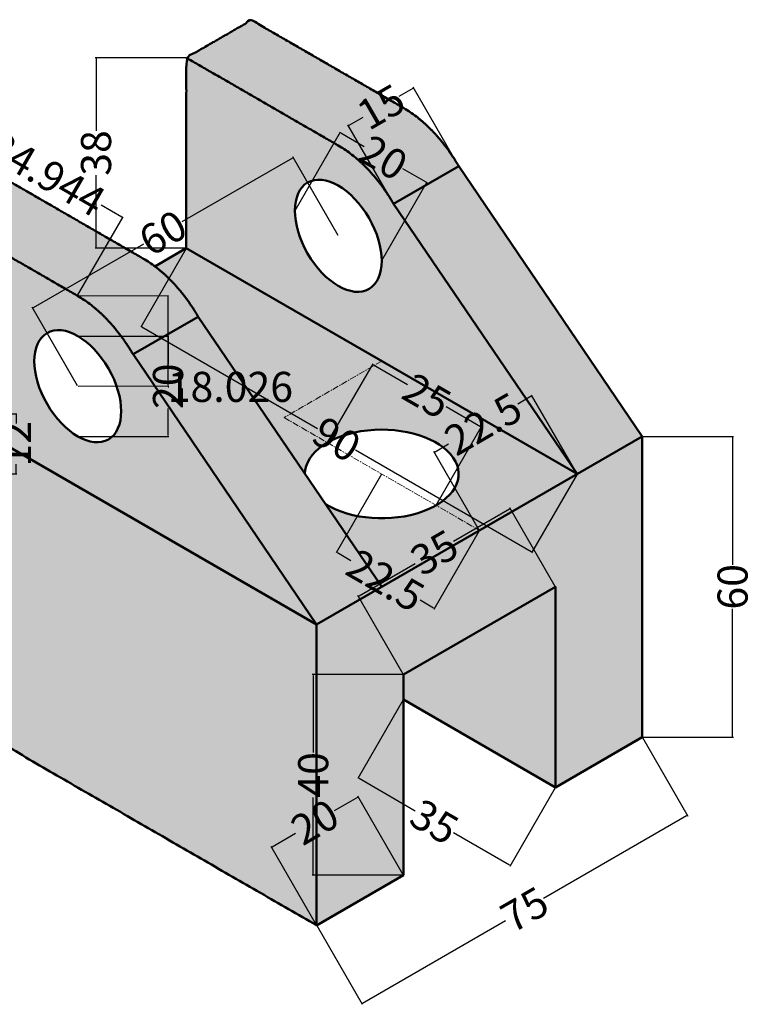
# Model space of a CAD drawing. Units: millimetres. Extents: x -57 to 165, y 2 to 198.
# Tile 1 of 1: x 18.8 to 164.9, y 1.8 to 198.1. Entities that reach past the tile are written whole.
import ezdxf

# ---------------------------------------------------------------- set-up
doc = ezdxf.new("R2010")
doc.units = ezdxf.units.MM
doc.header["$MEASUREMENT"] = 0
doc.linetypes.add('CENTER', pattern=[2, 1.25, -0.25, 0.25, -0.25])
for name, color, linetype, lineweight in [('M-CNTR', 7, 'CENTER', 18), ('M-DIMS', 2, 'Continuous', 18), ('M-HATC', 8, 'Continuous', 18), ('M-OUTL', 7, 'Continuous', 50)]:
    doc.layers.add(name, color=color, linetype=linetype, lineweight=lineweight)
doc.styles.get("Standard").update_dxf_attribs({"font": 'arial.ttf'})
doc.dimstyles.get("Standard").update_dxf_attribs({"dimtxt": 6, "dimasz": 0.18, "dimexe": 0.18, "dimexo": 0.0625, "dimgap": 0.09, "dimtad": 0, "dimtoh": 1, "dimdec": 0, "dimzin": 0, "dimdsep": 46, "dimtxsty": 'Standard', "dimcen": 0.09, "dimadec": 0, "dimazin": 0, "dimtfac": 1, "dimtdec": 0, "dimtofl": 0, "dimtmove": 0, "dimatfit": 3, "dimfxl": 1, "dimtolj": 1, "dimtzin": 0, "dimarcsym": 0})

# ---------------------------------------------------------------- blocks, each defined once
blk = doc.blocks.new('*D1')
at = {"layer": 'Defpoints', "color": 0, "transparency": 16777216}
for p in [(142.9404789999999, 54.99799699999999), (77.98857400000001, 17.497997), (86.98857372342155, 1.909540210928014)]:
    blk.add_point(p, dxfattribs=at)
at = {"layer": 'M-DIMS', "color": 0, "lineweight": -2, "transparency": 16777216}
for p, q in [((142.971729, 54.94387041226346), (152.0304787943798, 39.25365551534351)), ((151.7845942216985, 39.31954008802471), (123.2623607468992, 22.85222091346)), ((87.14445829610275, 1.999540210928017), (115.666691770902, 18.46685938549273)), ((78.01982400000001, 17.44387041226347), (87.07857372342156, 1.753655638246812))]:
    blk.add_line(p, q, dxfattribs=at)
at = {"layer": 'M-DIMS', "color": 0, "transparency": 16777216}
for points in [[(151.7695942216986, 39.34552085013825), (151.7995942216986, 39.29355932591118), (151.9404787943797, 39.40954008802471)], [(87.12945829610275, 2.025520973041551), (87.15945829610276, 1.973559448814484), (86.98857372342155, 1.909540210928014)]]:
    blk.add_solid(points, dxfattribs=at)
at = {"layer": 'M-DIMS', "color": 0, "transparency": 16777216, "insert": (119.4645262589006, 20.65954014947636), "char_height": 6, "attachment_point": 5, "rotation": 29.99999999999997}
blk.add_mtext('\\A1;75', dxfattribs=at)
blk = doc.blocks.new('*D2')
at = {"layer": 'Defpoints', "color": 0, "transparency": 16777216}
for p in [(52.007811, 152.497997), (43.00781132352439, 136.9095402922407), (129.9500979999999, 107.497997)]:
    blk.add_point(p, dxfattribs=at)
at = {"layer": 'M-DIMS', "color": 0, "lineweight": -2, "transparency": 16777216}
for p, q in [((51.976561, 152.4438704122635), (42.91781132352439, 136.7536557195595)), ((43.16369589620559, 136.8195402922407), (78.18820913771562, 116.5981281440193)), ((120.794213585993, 91.99954000671201), (85.76970034448304, 112.2209521549334)), ((129.9188479999999, 107.4438704122634), (120.8600981586743, 91.7536554340308))]:
    blk.add_line(p, q, dxfattribs=at)
at = {"layer": 'M-DIMS', "color": 0, "transparency": 16777216}
for points in [[(43.17869589620559, 136.8455210543543), (43.14869589620559, 136.7935595301272), (43.00781132352439, 136.9095402922407)], [(120.8092135859931, 92.02552076882554), (120.7792135859931, 91.97355924459848), (120.9500981586743, 91.909540006712)]]:
    blk.add_solid(points, dxfattribs=at)
at = {"layer": 'M-DIMS', "color": 0, "transparency": 16777216, "insert": (81.97895474109932, 114.4095401494764), "char_height": 6, "attachment_point": 5, "rotation": 330}
blk.add_mtext('\\A1;90', dxfattribs=at)
blk = doc.blocks.new('*D3')
at = {"layer": 'Defpoints', "color": 0, "transparency": 16777216}
for p in [(142.940479, 114.997997), (142.940479, 54.99799700000003), (160.9404790000001, 54.99799700000004)]:
    blk.add_point(p, dxfattribs=at)
at = {"layer": 'M-DIMS', "color": 0, "lineweight": -2, "transparency": 16777216}
for p, q in [((143.002979, 114.997997), (161.1204790000001, 114.997997)), ((160.9404790000001, 114.817997), (160.9404790000001, 89.39154406684862)), ((160.9404790000001, 55.17799700000003), (160.9404790000001, 80.60444993315147)), ((143.002979, 54.99799700000003), (161.1204790000001, 54.99799700000004))]:
    blk.add_line(p, q, dxfattribs=at)
at = {"layer": 'M-DIMS', "color": 0, "transparency": 16777216}
for points in [[(160.9104790000001, 114.817997), (160.9704790000001, 114.817997), (160.9404790000001, 114.997997)], [(160.9104790000001, 55.17799700000003), (160.9704790000001, 55.17799700000003), (160.9404790000001, 54.99799700000004)]]:
    blk.add_solid(points, dxfattribs=at)
at = {"layer": 'M-DIMS', "color": 0, "transparency": 16777216, "insert": (160.9404790000001, 84.99799699999996), "char_height": 6, "attachment_point": 5, "rotation": 90}
blk.add_mtext('\\A1;60', dxfattribs=at)
blk = doc.blocks.new('*D4')
at = {"layer": 'Defpoints', "color": 0, "transparency": 16777216}
for p in [(77.30908200000006, 67.49799700000003), (95.30908200000005, 67.49799700000003), (95.30908200000005, 27.49799700000002)]:
    blk.add_point(p, dxfattribs=at)
at = {"layer": 'M-DIMS', "color": 0, "lineweight": -2, "transparency": 16777216}
for p, q in [((95.24658200000002, 67.49799700000003), (77.12908200000007, 67.49799700000003)), ((77.30908200000006, 67.31799700000002), (77.30908200000006, 51.99590968758528)), ((77.30908200000007, 27.67799700000001), (77.30908200000006, 43.00008431241475)), ((95.24658200000002, 27.49799700000002), (77.12908200000008, 27.49799700000001))]:
    blk.add_line(p, q, dxfattribs=at)
at = {"layer": 'M-DIMS', "color": 0, "transparency": 16777216}
for points in [[(77.27908200000006, 67.31799700000002), (77.33908200000006, 67.31799700000002), (77.30908200000006, 67.49799700000003)], [(77.27908200000007, 27.67799700000001), (77.33908200000008, 27.67799700000001), (77.30908200000007, 27.49799700000001)]]:
    blk.add_solid(points, dxfattribs=at)
at = {"layer": 'M-DIMS', "color": 0, "transparency": 16777216, "insert": (77.30908200000006, 47.49799699999998), "char_height": 6, "attachment_point": 5, "rotation": 90}
blk.add_mtext('\\A1;40', dxfattribs=at)
blk = doc.blocks.new('*D5')
at = {"layer": 'Defpoints', "color": 0, "transparency": 16777216}
for p in [(116.6199710076562, 100.5864542548589), (125.619971, 84.99799699999998), (95.309082, 67.497997)]:
    blk.add_point(p, dxfattribs=at)
at = {"layer": 'M-DIMS', "color": 0, "lineweight": -2, "transparency": 16777216}
for p, q in [((116.464086434975, 100.4964542548589), (105.2818554117888, 94.04039016348177)), ((125.588721, 85.0521235877365), (116.5299710076562, 100.7423388275401)), ((86.4649665472236, 83.17645431221374), (97.6471975704098, 89.6325184035909)), ((95.277832, 67.5521235877365), (86.2190819745424, 83.24233888489493))]:
    blk.add_line(p, q, dxfattribs=at)
at = {"layer": 'M-DIMS', "color": 0, "transparency": 16777216}
for points in [[(116.449086434975, 100.5224350169724), (116.479086434975, 100.4704734927453), (116.6199710076562, 100.5864542548589)], [(86.4499665472236, 83.20243507432728), (86.4799665472236, 83.15047355010022), (86.3090819745424, 83.08645431221373)]]:
    blk.add_solid(points, dxfattribs=at)
at = {"layer": 'M-DIMS', "color": 0, "transparency": 16777216, "insert": (101.4645264910993, 91.83645428353631), "char_height": 6, "attachment_point": 5, "rotation": 30.000000000000025}
blk.add_mtext('\\A1;35', dxfattribs=at)
blk = doc.blocks.new('*D6')
at = {"layer": 'Defpoints', "color": 0, "transparency": 16777216}
for p in [(86.30908212556041, 43.08645405064289), (95.309082, 27.497997), (77.98857399999999, 17.497997)]:
    blk.add_point(p, dxfattribs=at)
at = {"layer": 'M-DIMS', "color": 0, "lineweight": -2, "transparency": 16777216}
for p, q in [((95.277832, 27.55212358773653), (86.2190821255604, 43.24233862332408)), ((86.1531975528792, 42.99645405064288), (81.483879248326, 40.30062187057703)), ((69.14445867931941, 33.17645408341707), (73.8137769838726, 35.87228626348291)), ((77.95732399999999, 17.55212358773652), (68.89857410663821, 33.24233865609827))]:
    blk.add_line(p, q, dxfattribs=at)
at = {"layer": 'M-DIMS', "color": 0, "transparency": 16777216}
for points in [[(86.1381975528792, 43.02243481275641), (86.1681975528792, 42.97047328852935), (86.30908212556041, 43.08645405064289)], [(69.12945867931943, 33.2024348455306), (69.15945867931941, 33.15047332130354), (68.98857410663821, 33.08645408341707)]]:
    blk.add_solid(points, dxfattribs=at)
at = {"layer": 'M-DIMS', "color": 0, "transparency": 16777216, "insert": (77.64882811609931, 38.08645406702998), "char_height": 6, "attachment_point": 5, "rotation": 30.000000000000025}
blk.add_mtext('\\A1;20', dxfattribs=at)
blk = doc.blocks.new('*D7')
at = {"layer": 'Defpoints', "color": 0, "transparency": 16777216}
for p in [(95.30908199999998, 62.497997), (86.30908197454241, 46.90953968778624), (125.619971, 44.99799699999999)]:
    blk.add_point(p, dxfattribs=at)
at = {"layer": 'M-DIMS', "color": 0, "lineweight": -2, "transparency": 16777216}
for p, q in [((95.277832, 62.44387041226346), (86.2190819745424, 46.75365511510503)), ((86.4649665472236, 46.81953968778624), (97.64719757040984, 40.3634755964091)), ((125.588721, 44.94387041226346), (116.5299710076562, 29.2536551724599)), ((116.464086434975, 29.49953974514112), (105.2818554117888, 35.95560383651826))]:
    blk.add_line(p, q, dxfattribs=at)
at = {"layer": 'M-DIMS', "color": 0, "transparency": 16777216}
for points in [[(86.4799665472236, 46.84552044989978), (86.4499665472236, 46.79355892567271), (86.30908197454241, 46.90953968778624)], [(116.479086434975, 29.52552050725465), (116.449086434975, 29.47355898302759), (116.6199710076562, 29.40953974514112)]]:
    blk.add_solid(points, dxfattribs=at)
at = {"layer": 'M-DIMS', "color": 0, "transparency": 16777216, "insert": (101.4645264910993, 38.15953971646368), "char_height": 6, "attachment_point": 5, "rotation": 330}
blk.add_mtext('\\A1;35', dxfattribs=at)
blk = doc.blocks.new('*D8')
at = {"layer": 'Defpoints', "color": 0, "transparency": 16777216}
for p in [(34.00781100000002, 190.497997), (52.00781100000003, 190.497997), (52.00781100000003, 152.497997)]:
    blk.add_point(p, dxfattribs=at)
at = {"layer": 'M-DIMS', "color": 0, "lineweight": -2, "transparency": 16777216}
for p, q in [((51.94531100000002, 190.497997), (33.82781100000002, 190.497997)), ((34.00781100000002, 190.317997), (34.00781100000003, 175.8894976821283)), ((34.00781100000003, 152.677997), (34.00781100000003, 167.1064963178718)), ((51.94531100000002, 152.497997), (33.82781100000002, 152.497997))]:
    blk.add_line(p, q, dxfattribs=at)
at = {"layer": 'M-DIMS', "color": 0, "transparency": 16777216}
for points in [[(33.97781100000002, 190.317997), (34.03781100000002, 190.317997), (34.00781100000002, 190.497997)], [(33.97781100000003, 152.677997), (34.03781100000003, 152.677997), (34.00781100000003, 152.497997)]]:
    blk.add_solid(points, dxfattribs=at)
at = {"layer": 'M-DIMS', "color": 0, "transparency": 16777216, "insert": (34.00781100000006, 171.497997), "char_height": 6, "attachment_point": 5, "rotation": 90}
blk.add_mtext('\\A1;38', dxfattribs=at)
blk = doc.blocks.new('*D9')
at = {"layer": 'Defpoints', "color": 0, "transparency": 16777216}
for p in [(97.33178524819515, 184.4504148382333), (106.331785, 168.861958), (93.341404, 161.3619579999999)]:
    blk.add_point(p, dxfattribs=at)
at = {"layer": 'M-DIMS', "color": 0, "lineweight": -2, "transparency": 16777216}
for p, q in [((106.300535, 168.9160845877365), (97.24178524819514, 184.6062994109145)), ((97.17590067551393, 184.3604148382333), (94.41112936372917, 182.7641733771266)), ((93.310154, 161.4160845877365), (84.25140423400347, 177.1062994354951)), ((84.49728880668468, 177.0404148628139), (87.2620601184694, 178.6366563239206))]:
    blk.add_line(p, q, dxfattribs=at)
at = {"layer": 'M-DIMS', "color": 0, "transparency": 16777216}
for points in [[(97.16090067551391, 184.3863956003468), (97.19090067551392, 184.3344340761197), (97.33178524819515, 184.4504148382333)], [(84.48228880668466, 177.0663956249274), (84.51228880668467, 177.0144341007004), (84.34140423400348, 176.9504148628139)]]:
    blk.add_solid(points, dxfattribs=at)
at = {"layer": 'M-DIMS', "color": 0, "transparency": 16777216, "insert": (90.8365947410993, 180.7004148505236), "char_height": 6, "attachment_point": 5, "rotation": 30.000000000000053}
blk.add_mtext('\\A1;15', dxfattribs=at)
blk = doc.blocks.new('*D10')
at = {"layer": 'Defpoints', "color": 0, "transparency": 16777216}
for p in [(73.31870089448267, 170.5864544508813), (82.318701, 154.997997), (30.35717600000001, 124.997997)]:
    blk.add_point(p, dxfattribs=at)
at = {"layer": 'M-DIMS', "color": 0, "lineweight": -2, "transparency": 16777216}
for p, q in [((73.16281632180147, 170.4964544508813), (51.14286186371283, 157.7832278169606)), ((82.28745099999999, 155.0521235877365), (73.22870089448267, 170.7423390235625)), ((21.51306066039725, 140.6764541161913), (43.53301511848588, 153.389680750112)), ((30.32592600000001, 125.0521235877365), (21.26717608771604, 140.7423386888725))]:
    blk.add_line(p, q, dxfattribs=at)
at = {"layer": 'M-DIMS', "color": 0, "transparency": 16777216}
for points in [[(73.14781632180149, 170.5224352129948), (73.17781632180149, 170.4704736887677), (73.31870089448267, 170.5864544508813)], [(21.49806066039725, 140.7024348783048), (21.52806066039725, 140.6504733540778), (21.35717608771605, 140.5864541161913)]]:
    blk.add_solid(points, dxfattribs=at)
at = {"layer": 'M-DIMS', "color": 0, "transparency": 16777216, "insert": (47.33793849109936, 155.5864542835363), "char_height": 6, "attachment_point": 5, "rotation": 29.999999999999883}
blk.add_mtext('\\A1;60', dxfattribs=at)
blk = doc.blocks.new('*D11')
at = {"layer": 'Defpoints', "color": 0, "transparency": 16777216}
for p in [(99.97895489336175, 165.586454083417), (73.658447, 159.997997), (90.97895499999998, 149.997997)]:
    blk.add_point(p, dxfattribs=at)
at = {"layer": 'M-DIMS', "color": 0, "lineweight": -2, "transparency": 16777216}
for p, q in [((73.689697, 160.0521235877365), (82.74844687443955, 175.742338623324)), ((82.81433144712074, 175.4964540506428), (87.48364975167397, 172.800621870577)), ((99.82307032068054, 165.676454083417), (95.15375201612736, 168.3722862634828)), ((91.01020499999998, 150.0521235877365), (100.0689548933617, 165.7423386560982))]:
    blk.add_line(p, q, dxfattribs=at)
at = {"layer": 'M-DIMS', "color": 0, "transparency": 16777216}
for points in [[(82.82933144712075, 175.5224348127563), (82.79933144712074, 175.4704732885293), (82.65844687443955, 175.5864540506428)], [(99.83807032068054, 165.7024348455306), (99.80807032068056, 165.6504733213035), (99.97895489336175, 165.586454083417)]]:
    blk.add_solid(points, dxfattribs=at)
at = {"layer": 'M-DIMS', "color": 0, "transparency": 16777216, "insert": (91.31870088390065, 170.5864540670299), "char_height": 6, "attachment_point": 5, "rotation": 330}
blk.add_mtext('\\A1;20', dxfattribs=at)
blk = doc.blocks.new('*D12')
at = {"layer": 'Defpoints', "color": 0, "transparency": 16777216}
for p in [(30.35717600000002, 134.997997), (30.35717600000002, 114.997997), (48.35717600000005, 114.997997)]:
    blk.add_point(p, dxfattribs=at)
at = {"layer": 'M-DIMS', "color": 0, "lineweight": -2, "transparency": 16777216}
for p, q in [((30.41967600000001, 134.997997), (48.53717600000006, 134.997997)), ((48.35717600000005, 134.817997), (48.35717600000005, 129.4263326070942)), ((48.35717600000005, 115.1779970000001), (48.35717600000005, 120.5696613929059)), ((30.41967600000001, 114.997997), (48.53717600000006, 114.997997))]:
    blk.add_line(p, q, dxfattribs=at)
at = {"layer": 'M-DIMS', "color": 0, "transparency": 16777216}
for points in [[(48.32717600000005, 134.817997), (48.38717600000006, 134.817997), (48.35717600000005, 134.997997)], [(48.32717600000005, 115.1779970000001), (48.38717600000006, 115.1779970000001), (48.35717600000005, 114.997997)]]:
    blk.add_solid(points, dxfattribs=at)
at = {"layer": 'M-DIMS', "color": 0, "transparency": 16777216, "insert": (48.35717600000008, 124.997997), "char_height": 6, "attachment_point": 5, "rotation": 90}
blk.add_mtext('\\A1;20', dxfattribs=at)
blk = doc.blocks.new('*D14')
at = {"layer": 'Defpoints', "color": 0, "transparency": 16777216}
for p in [(110.804272020727, 116.8364543040202), (80.15363699999999, 113.747997), (101.804272, 101.247997)]:
    blk.add_point(p, dxfattribs=at)
at = {"layer": 'M-DIMS', "color": 0, "lineweight": -2, "transparency": 16777216}
for p, q in [((80.184887, 113.8021235877365), (89.24363699707429, 129.4923388357336)), ((89.30952156975547, 129.2464542630524), (96.11554783821445, 125.316993164846)), ((110.6483874480458, 116.9264543040202), (103.8423611795868, 120.8559154022266)), ((101.835522, 101.3021235877365), (110.894272020727, 116.9923388767014))]:
    blk.add_line(p, q, dxfattribs=at)
at = {"layer": 'M-DIMS', "color": 0, "transparency": 16777216}
for points in [[(89.32452156975548, 129.272435025166), (89.29452156975547, 129.2204735009389), (89.15363699707429, 129.3364542630524)], [(110.6633874480458, 116.9524350661337), (110.6333874480458, 116.9004735419066), (110.804272020727, 116.8364543040202)]]:
    blk.add_solid(points, dxfattribs=at)
at = {"layer": 'M-DIMS', "color": 0, "transparency": 16777216, "insert": (99.97895450890066, 123.0864542835363), "char_height": 6, "attachment_point": 5, "rotation": 330}
blk.add_mtext('\\A1;25', dxfattribs=at)
blk = doc.blocks.new('*D15')
at = {"layer": 'Defpoints', "color": 0, "transparency": 16777216}
for p in [(90.97895499999998, 107.497997), (110.464526, 96.247997), (81.97895491795558, 91.909539589775)]:
    blk.add_point(p, dxfattribs=at)
at = {"layer": 'M-DIMS', "color": 0, "lineweight": -2, "transparency": 16777216}
for p, q in [((90.947705, 107.4438704122634), (81.88895491795557, 91.75365501709379)), ((110.433276, 96.19387041226346), (101.374526064243, 80.50365527047111)), ((82.13483949063676, 91.819539589775), (84.83138008985958, 90.26269114893294)), ((101.3086414915618, 80.74953984315232), (98.61210089233907, 82.30638828399435))]:
    blk.add_line(p, q, dxfattribs=at)
at = {"layer": 'M-DIMS', "color": 0, "transparency": 16777216}
for points in [[(82.14983949063677, 91.84552035188854), (82.11983949063676, 91.79355882766146), (81.97895491795558, 91.909539589775)], [(101.3236414915618, 80.77552060526585), (101.2936414915619, 80.72355908103879), (101.464526064243, 80.65953984315232)]]:
    blk.add_solid(points, dxfattribs=at)
at = {"layer": 'M-DIMS', "color": 0, "transparency": 16777216, "insert": (91.72174049109933, 86.28453971646366), "char_height": 6, "attachment_point": 5, "rotation": 330}
blk.add_mtext('\\A1;22.5', dxfattribs=at)
blk = doc.blocks.new('*D16')
at = {"layer": 'Defpoints', "color": 0, "transparency": 16777216}
for p in [(120.9500980642432, 123.0864541568477), (129.950098, 107.497997), (110.464526, 96.247997)]:
    blk.add_point(p, dxfattribs=at)
at = {"layer": 'M-DIMS', "color": 0, "lineweight": -2, "transparency": 16777216}
for p, q in [((120.794213491562, 122.9964541568477), (118.0976725173392, 121.4396054994993)), ((129.918848, 107.5521235877365), (120.8600980642432, 123.2423387295288)), ((110.433276, 96.30212358773655), (101.3745261679557, 111.9923385498936)), ((101.6204107406369, 111.9264539772125), (104.3169517148597, 113.4833026345608))]:
    blk.add_line(p, q, dxfattribs=at)
at = {"layer": 'M-DIMS', "color": 0, "transparency": 16777216}
for points in [[(120.779213491562, 123.0224349189612), (120.809213491562, 122.9704733947341), (120.9500980642432, 123.0864541568477)], [(101.6054107406369, 111.952434739326), (101.6354107406369, 111.9004732150989), (101.4645261679557, 111.8364539772124)]]:
    blk.add_solid(points, dxfattribs=at)
at = {"layer": 'M-DIMS', "color": 0, "transparency": 16777216, "insert": (111.2073121160994, 117.4614540670301), "char_height": 6, "attachment_point": 5, "rotation": 29.999999999999538}
blk.add_mtext('\\A1;22.5', dxfattribs=at)
blk = doc.blocks.new('*D17')
at = {"layer": 'Defpoints', "color": 0, "transparency": 16777216}
for p in [(0.0462869999999924, 160.497997), (39.30844832468702, 158.6118924312673), (30.307407, 143.024036)]:
    blk.add_point(p, dxfattribs=at)
at = {"layer": 'M-DIMS', "color": 0, "lineweight": -2, "transparency": 16777216}
for p, q in [((0.0775406150812756, 160.5521215004074), (9.137338633268897, 176.2417318143229)), ((9.203206783008142, 175.9958428417155), (13.32703206028853, 173.6145839495605)), ((39.1525697635137, 158.7019028427014), (35.0287444862333, 161.0831617348563)), ((30.33866061508128, 143.0781605004074), (39.39845873612112, 158.7677709924407))]:
    blk.add_line(p, q, dxfattribs=at)
at = {"layer": 'M-DIMS', "color": 0, "transparency": 16777216}
for points in [[(9.218208518247167, 176.021822601911), (9.18820504776913, 175.9698630815199), (9.047328221834803, 176.0858532531495)], [(39.16757149875272, 158.727882602897), (39.13756802827469, 158.6759230825059), (39.30844832468702, 158.6118924312673)]]:
    blk.add_solid(points, dxfattribs=at)
at = {"layer": 'M-DIMS', "color": 0, "transparency": 16777216, "insert": (24.17788827326091, 167.3488728422084), "char_height": 6, "attachment_point": 5, "rotation": 329.9961731765761}
blk.add_mtext('\\A1;34.944', dxfattribs=at)
blk = doc.blocks.new('*D18')
at = {"layer": 'Defpoints', "color": 0, "transparency": 16777216}
for p in [(30.307407, 143.024036), (30.357176, 124.997997), (48.35710765869329, 125.0476942343873)]:
    blk.add_point(p, dxfattribs=at)
at = {"layer": 'M-DIMS', "color": 0, "lineweight": -2, "transparency": 16777216}
for p, q in [((30.36990676178436, 143.0242085598391), (48.48733765671476, 143.0742302058516)), ((48.30783531511237, 142.8937339195761), (48.35661068635673, 125.2276935483263)), ((30.41967576178436, 124.998169559839), (48.53710697263225, 125.0481912067239)), ((48.35710765869329, 125.0476942343873), (48.35760463102985, 124.8676949204483)), ((48.35760463102985, 124.8676949204483), (48.53760463102986, 124.8676949204483))]:
    blk.add_line(p, q, dxfattribs=at)
at = {"layer": 'M-DIMS', "color": 0, "transparency": 16777216}
for points in [[(48.33783520076885, 142.8938167482989), (48.27783542945587, 142.8936510908533), (48.3073383427758, 143.073733233515)], [(48.38661057201322, 125.227776377049), (48.32661080070024, 125.2276107196035), (48.35710765869329, 125.0476942343873)]]:
    blk.add_solid(points, dxfattribs=at)
at = {"layer": 'M-DIMS', "color": 0, "transparency": 16777216, "insert": (60.79745456281703, 124.8676949204483), "char_height": 6, "attachment_point": 5}
blk.add_mtext('\\A1;18.026', dxfattribs=at)
blk = doc.blocks.new('*D19')
at = {"layer": 'Defpoints', "color": 0, "transparency": 16777216}
for p in [(0.046287, 119.497997), (0.046287, 107.497997), (18.04628700000001, 107.497997)]:
    blk.add_point(p, dxfattribs=at)
at = {"layer": 'M-DIMS', "color": 0, "lineweight": -2, "transparency": 16777216}
for p, q in [((0.108787, 119.497997), (18.22628700000001, 119.497997)), ((18.04628700000001, 119.317997), (18.04628700000001, 117.5723080504775)), ((18.04628700000001, 107.677997), (18.04628700000001, 109.4236859495225)), ((0.108787, 107.497997), (18.22628700000001, 107.497997))]:
    blk.add_line(p, q, dxfattribs=at)
at = {"layer": 'M-DIMS', "color": 0, "transparency": 16777216}
for points in [[(18.01628700000001, 119.317997), (18.07628700000001, 119.317997), (18.04628700000001, 119.497997)], [(18.01628700000001, 107.677997), (18.07628700000001, 107.677997), (18.04628700000001, 107.497997)]]:
    blk.add_solid(points, dxfattribs=at)
at = {"layer": 'M-DIMS', "color": 0, "transparency": 16777216, "insert": (18.04628700000004, 113.497997), "char_height": 6, "attachment_point": 5, "rotation": 90}
blk.add_mtext('\\A1;12', dxfattribs=at)

msp = doc.modelspace()

# ---------------------------------------------------------------- hatches: boundary and pattern name
at = {"layer": 'M-HATC'}
h = msp.add_hatch(color=256, dxfattribs=at)
h.set_gradient(color1=(16, 86, 137), color2=(147, 149, 152), tint=1)
h.paths.add_polyline_path([(95.30908161067455, 67.49799706451296), (125.6199707431299, 84.99799706451296), (125.6199707431299, 44.99799706451294), (142.9404788188187, 54.99799706451296), (142.9404788188187, 114.9979970645127), (77.98857353498579, 77.49799706451294), (77.98857353498579, 17.49799706451294), (95.30908161067455, 27.49799706451294)])
edge = h.paths.add_edge_path()
edge.add_spline(control_points=[(41.37988016936596, 131.3619580951918), (36.81412674377037, 139.2700750031551), (30.35717632684165, 142.9979970645129)], knot_values=[0, 0, 0, 0.7853981633974488, 0.7853981633974488, 0.7853981633974488], weights=[1, 0.9238795325112866, 1], degree=2, periodic=0)
edge.add_spline(control_points=[(30.35717632684165, 142.9979970645129), (15.20173176061398, 151.7479970645129), (0.0462871943863021, 160.4979970645129)], knot_values=[0.7853981633974488, 0.7853981633974488, 0.7853981633974488, 1.785398163397448, 1.785398163397448, 1.785398163397448], weights=[1, 1, 1], degree=2, periodic=0)
edge.add_spline(control_points=[(0.046287194386295, 160.4979970645129), (0.046287194386295, 147.4979970645129), (0.046287194386295, 134.4979970645129)], knot_values=[2.785398163397448, 2.785398163397448, 2.785398163397448, 3.419544504860864, 3.419544504860864, 3.419544504860864], weights=[1, 1, 1], degree=2, periodic=0)
edge.add_spline(control_points=[(0.046287194386295, 134.4979970645129), (0.046287194386295, 126.9979970645129), (0.046287194386295, 119.4979970645129)], knot_values=[3.419544504860864, 3.419544504860864, 3.419544504860864, 3.785398163397448, 3.785398163397448, 3.785398163397448], weights=[1, 1, 1], degree=2, periodic=0)
edge.add_spline(control_points=[(0.046287194386295, 119.4979970645129), (6.541477722769585, 123.2479970645129), (13.03666825115288, 126.9979970645129)], knot_values=[3, 3, 3, 4, 4, 4], weights=[1, 1, 1], degree=2, periodic=0)
edge.add_spline(control_points=[(13.03666825115288, 126.9979970645129), (13.03666825115288, 90.99799706451292), (13.03666825115288, 54.99799706451296)], knot_values=[2, 2, 2, 3, 3, 3], weights=[1, 1, 1], degree=2, periodic=0)
edge.add_line((13.03666825115287, 114.9979970645129), (77.98857353498579, 77.49799706451294))
edge.add_line((77.98857353498579, 77.49799706451294), (41.37988016936608, 131.3619580951916))
edge = h.paths.add_edge_path(flags=16)
edge.add_ellipse((30.35717632684166, 124.9979970645129), major_axis=(6.123724356957944, -10.60660171779821), ratio=0.577350269189626, start_angle=0, end_angle=360)
h.paths.add_polyline_path([(54.37026122613253, 138.8619580951918), (41.37988016936596, 131.3619580951918), (77.98857353498579, 77.49799706451294), (90.97895459175238, 84.99799706451292)])
edge = h.paths.add_edge_path()
edge.add_spline(control_points=[(45.75812342050349, 148.8897380148136), (44.56013330857391, 149.7979160278211), (43.34755738360823, 150.4979970645129)], knot_values=[0.6281854185381637, 0.6281854185381637, 0.6281854185381637, 0.7853981633974488, 0.7853981633974488, 0.7853981633974488], weights=[0.975625973363323, 0.9847630053244513, 1], degree=2, periodic=0)
edge.add_spline(control_points=[(43.34755738360823, 150.4979970645129), (28.19211281738056, 159.2479970645129), (13.03666825115287, 167.9979970645129)], knot_values=[0.7853981633974488, 0.7853981633974488, 0.7853981633974488, 1.785398163397448, 1.785398163397448, 1.785398163397448], weights=[1, 1, 1], degree=2, periodic=0)
edge.add_spline(control_points=[(13.03666825115287, 167.9979970645129), (6.541477722769585, 164.2479970645129), (0.046287194386295, 160.4979970645129)], knot_values=[1.785398163397448, 1.785398163397448, 1.785398163397448, 2.785398163397448, 2.785398163397448, 2.785398163397448], weights=[1, 1, 1], degree=2, periodic=0)
edge.add_spline(control_points=[(0.0462871943863021, 160.4979970645129), (15.20173176061398, 151.7479970645129), (30.35717632684165, 142.9979970645129)], knot_values=[0.7853981633974488, 0.7853981633974488, 0.7853981633974488, 1.785398163397448, 1.785398163397448, 1.785398163397448], weights=[1, 1, 1], degree=2, periodic=0)
edge.add_spline(control_points=[(30.35717632684165, 142.9979970645129), (36.81412674377037, 139.2700750031551), (41.37988016936596, 131.3619580951918)], knot_values=[0, 0, 0, 0.7853981633974488, 0.7853981633974488, 0.7853981633974488], weights=[1, 0.9238795325112866, 1], degree=2, periodic=0)
edge.add_line((41.37988016936598, 131.3619580951918), (54.37026122613254, 138.8619580951918))
edge.add_spline(control_points=[(54.37026122613254, 138.8619580951918), (50.7776825657607, 145.0844868651436), (45.75812342050349, 148.8897380148136)], knot_values=[0, 0, 0, 0.6281854185381637, 0.6281854185381637, 0.6281854185381637], weights=[1, 0.9391165271868352, 0.975625973363323], degree=2, periodic=0)
edge = h.paths.add_edge_path()
edge.add_spline(control_points=[(95.30908161067462, 180.4979970645128), (80.15363704444697, 189.2479970645128), (64.9981924782193, 197.9979970645128)], knot_values=[0.7853981633974488, 0.7853981633974488, 0.7853981633974488, 1.785398163397448, 1.785398163397448, 1.785398163397448], weights=[1, 1, 1], degree=2, periodic=0)
edge.add_spline(control_points=[(64.9981924782193, 197.9979970645128), (58.503001949836, 194.2479970645128), (52.0078114214527, 190.4979970645127)], knot_values=[1.785398163397448, 1.785398163397448, 1.785398163397448, 2.785398163397447, 2.785398163397448, 2.785398163397448], weights=[1, 1, 1], degree=2, periodic=0)
edge.add_spline(control_points=[(52.00781142145273, 190.4979970645127), (67.1632559876804, 181.7479970645128), (82.31870055390804, 172.9979970645128)], knot_values=[0.7853981633974488, 0.7853981633974488, 0.7853981633974488, 1.785398163397448, 1.785398163397448, 1.785398163397448], weights=[1, 1, 1], degree=2, periodic=0)
edge.add_spline(control_points=[(82.31870055390804, 172.9979970645128), (88.77565097083676, 169.2700750031549), (93.34140439643235, 161.3619580951917)], knot_values=[0, 0, 0, 0.7853981633974488, 0.7853981633974488, 0.7853981633974488], weights=[1, 0.9238795325112866, 1], degree=2, periodic=0)
edge.add_line((93.34140439643235, 161.3619580951917), (106.3317854531989, 168.8619580951917))
edge.add_spline(control_points=[(106.3317854531989, 168.8619580951917), (101.7660320276033, 176.7700750031549), (95.30908161067462, 180.4979970645128)], knot_values=[0, 0, 0, 0.7853981633974488, 0.7853981633974488, 0.7853981633974488], weights=[1, 0.9238795325112866, 1], degree=2, periodic=0)
h.paths.add_polyline_path([(106.3317854531989, 168.8619580951917), (93.34140439643235, 161.3619580951917), (129.9500977620521, 107.4979970645128), (142.9404788188187, 114.9979970645128)])
edge = h.paths.add_edge_path()
edge.add_spline(control_points=[(93.34140439643235, 161.3619580951917), (88.77565097083676, 169.2700750031549), (82.31870055390804, 172.9979970645128)], knot_values=[0, 0, 0, 0.7853981633974488, 0.7853981633974488, 0.7853981633974488], weights=[1, 0.9238795325112866, 1], degree=2, periodic=0)
edge.add_spline(control_points=[(82.31870055390804, 172.9979970645128), (67.1632559876804, 181.7479970645128), (52.00781142145273, 190.4979970645127)], knot_values=[0.7853981633974488, 0.7853981633974488, 0.7853981633974488, 1.785398163397448, 1.785398163397448, 1.785398163397448], weights=[1, 1, 1], degree=2, periodic=0)
edge.add_spline(control_points=[(52.0078114214527, 190.4979970645127), (52.0078114214527, 171.4979970645128), (52.0078114214527, 152.4979970645128)], knot_values=[2.785398163397447, 2.785398163397448, 2.785398163397448, 3.785398163397448, 3.785398163397448, 3.785398163397448], weights=[1, 1, 1], degree=2, periodic=0)
edge.add_line((52.0078114214527, 152.4979970645128), (129.9500977620521, 107.4979970645128))
edge.add_line((129.9500977620521, 107.4979970645128), (93.34140439643232, 161.3619580951917))
edge = h.paths.add_edge_path(flags=16)
edge.add_ellipse((82.31870055390804, 154.9979970645128), major_axis=(6.123724356957944, -10.60660171779821), ratio=0.577350269189626, start_angle=0, end_angle=360)
edge = h.paths.add_edge_path()
edge.add_line((52.0078114214527, 152.4979970645128), (45.7581234205035, 148.8897380148136))
edge.add_spline(control_points=[(45.75812342050349, 148.8897380148136), (50.7776825657607, 145.0844868651436), (54.37026122613254, 138.8619580951918)], knot_values=[0, 0, 0, 0.6281854185381637, 0.6281854185381637, 0.6281854185381637], weights=[0.975625973363323, 0.9391165271868352, 1], degree=2, periodic=0)
edge.add_line((54.37026122613257, 138.8619580951917), (75.66970573764932, 107.5231600210469))
edge.add_ellipse((90.97895459175238, 107.4979970645129), major_axis=(-15.30931089239486, 0), ratio=0.577350269189626, start_angle=330, end_angle=359.90582621493047, ccw=False)
edge.add_line((80.1536370444469, 113.7479970645129), (71.49338300660253, 118.7479970645128))
edge.add_line((71.49338300660253, 118.7479970645128), (90.97895459175236, 129.9979970645128))
edge.add_line((90.97895459175236, 129.9979970645128), (52.0078114214527, 152.4979970645128))
edge = h.paths.add_edge_path()
edge.add_line((90.97895459175236, 129.9979970645128), (71.49338300660254, 118.7479970645128))
edge.add_line((71.49338300660254, 118.7479970645128), (80.15363704444688, 113.7479970645129))
edge.add_ellipse((90.97895459175238, 107.4979970645129), major_axis=(-15.30931089239486, 0), ratio=0.577350269189626, start_angle=150.0000000000001, end_angle=330, ccw=False)
edge.add_line((101.8042721390579, 101.2479970645129), (110.4645261769023, 96.24799706451292))
edge.add_line((110.4645261769023, 96.24799706451292), (129.9500977620521, 107.4979970645128))
edge.add_line((129.9500977620521, 107.4979970645128), (90.97895459175236, 129.9979970645128))
edge = h.paths.add_edge_path(flags=17)
edge.add_line((110.4645261769023, 96.24799706451292), (101.8042721390579, 101.2479970645129))
edge.add_ellipse((90.97895459175238, 107.4979970645129), major_axis=(-15.30931089239486, 0), ratio=0.577350269189626, start_angle=28.308251316207816, end_angle=150.0000000000001, ccw=False)
edge.add_line((79.784778540041, 101.4684746256213), (90.97895459175238, 84.99799706451292))
edge.add_line((90.97895459175238, 84.99799706451292), (110.4645261769023, 96.24799706451292))
edge = h.paths.add_edge_path()
edge.add_line((77.98857353498579, 77.49799706451294), (13.03666825115287, 114.9979970645129))
edge.add_spline(control_points=[(13.03666825115288, 114.9979970645129), (13.03666825115288, 84.99799706451293), (13.03666825115288, 54.99799706451296)], knot_values=[2, 2, 2, 2.833333333333333, 2.833333333333333, 2.833333333333333], weights=[1, 1, 1], degree=2, periodic=0)
edge.add_spline(control_points=[(13.03666825115288, 54.99799706451296), (45.51262089306933, 36.24799706451295), (77.98857353498579, 17.49799706451294)], knot_values=[3.737462993461563, 3.737462993461563, 3.737462993461563, 4.570796326794897, 4.570796326794897, 4.570796326794897], weights=[1, 1, 1], degree=2, periodic=0)
edge.add_line((77.98857353498579, 17.49799706451294), (77.98857353498579, 77.49799706451294))
edge = h.paths.add_edge_path()
edge.add_spline(control_points=[(13.03666825115288, 54.99799706451296), (13.03666825115288, 84.99799706451293), (13.03666825115288, 114.9979970645129)], knot_values=[2, 2, 2, 2.833333333333333, 2.833333333333333, 2.833333333333333], weights=[1, 1, 1], degree=2, periodic=0)
edge.add_spline(control_points=[(13.03666825115288, 114.9979970645129), (13.03666825115288, 120.9979970645129), (13.03666825115288, 126.9979970645129)], knot_values=[2.833333333333333, 2.833333333333333, 2.833333333333333, 3, 3, 3], weights=[1, 1, 1], degree=2, periodic=0)
edge.add_spline(control_points=[(13.03666825115288, 126.9979970645129), (6.541477722769585, 123.2479970645129), (0.046287194386295, 119.4979970645129)], knot_values=[3, 3, 3, 4, 4, 4], weights=[1, 1, 1], degree=2, periodic=0)
edge.add_spline(control_points=[(0.046287194386295, 119.4979970645129), (-4.258346416899511, 117.0127156902743), (-7.302182033963242, 111.7406377516322), (-10.34601765102697, 106.46855981299), (-10.34601765102697, 101.4979970645129)], knot_values=[4, 4, 4, 4.785398163397448, 4.785398163397448, 5.570796326794897, 5.570796326794897, 5.570796326794897], weights=[1, 0.9238795325112866, 1, 0.9238795325112866, 1], degree=2, periodic=0)
edge.add_spline(control_points=[(-10.34601765102697, 101.4979970645129), (-9.046979545350315, 102.2479970645129), (-7.747941439673653, 102.9979970645129)], knot_values=[0.8749999999999998, 0.8749999999999998, 0.8749999999999998, 1, 1, 1], weights=[1, 1, 1], degree=2, periodic=0)
edge.add_ellipse((0.0462871943862933, 107.4979970645129), major_axis=(-5.511351921262146, -9.545941546018396), ratio=0.577350269189626, start_angle=150, end_angle=330, ccw=False)
edge.add_ellipse((0.0462871943862933, 107.4979970645129), major_axis=(-5.511351921262146, -9.545941546018396), ratio=0.577350269189626, start_angle=330, end_angle=509.9999999999999, ccw=False)
edge.add_spline(control_points=[(-7.747941439673653, 102.9979970645129), (-9.046979545350315, 102.2479970645129), (-10.34601765102697, 101.4979970645129)], knot_values=[0.8749999999999998, 0.8749999999999998, 0.8749999999999998, 1, 1, 1], weights=[1, 1, 1], degree=2, periodic=0)
edge.add_spline(control_points=[(-10.34601765102697, 101.4979970645129), (1.345325300062951, 78.24799706451296), (13.03666825115288, 54.99799706451296)], knot_values=[1, 1, 1, 2, 2, 2], weights=[1, 1, 1], degree=2, periodic=0)
edge = h.paths.add_edge_path()
edge.add_spline(control_points=[(0.046287194386295, 119.4979970645129), (0.046287194386295, 126.9979970645129), (0.046287194386295, 134.4979970645129)], knot_values=[3.419544504860864, 3.419544504860864, 3.419544504860864, 3.785398163397449, 3.785398163397449, 3.785398163397449], weights=[1, 1, 1], degree=2, periodic=0)
edge.add_spline(control_points=[(0.0462871943863093, 134.4979970645129), (-6.448903333996982, 130.7479970645129), (-12.94409386238027, 126.9979970645129)], knot_values=[0, 0, 0, 1, 1, 1], weights=[1, 1, 1], degree=2, periodic=0)
edge.add_spline(control_points=[(-12.94409386238027, 126.9979970645129), (-17.24872747366608, 124.5127156902743), (-20.29256309072981, 119.2406377516322), (-22.11694969149519, 116.0807074664587), (-22.87621616226442, 112.7950566133887)], knot_values=[1, 1, 1, 1.785398163397448, 1.785398163397448, 2.27095043198655, 2.27095043198655, 2.27095043198655], weights=[1, 0.9238795325112866, 1, 0.9529404735104989, 0.9640676373154162], degree=2, periodic=0)
edge.add_spline(control_points=[(-22.87621616226443, 112.7950566133887), (-23.10630743502899, 110.8965268389508), (-23.33639870779354, 108.9979970645129)], knot_values=[6.570796326794897, 6.570796326794897, 6.570796326794897, 7.570796326794897, 7.570796326794897, 7.570796326794897], weights=[1, 1, 1], degree=2, periodic=0)
edge.add_spline(control_points=[(-23.33639870779354, 108.9979970645129), (-16.84120817941026, 105.2479970645129), (-10.34601765102697, 101.4979970645129)], knot_values=[5.570796326794897, 5.570796326794897, 5.570796326794897, 6.570796326794897, 6.570796326794897, 6.570796326794897], weights=[1, 1, 1], degree=2, periodic=0)
edge.add_spline(control_points=[(-10.34601765102697, 101.4979970645129), (-10.34601765102697, 106.46855981299), (-7.302182033963242, 111.7406377516322), (-4.258346416899511, 117.0127156902743), (0.046287194386295, 119.4979970645129)], knot_values=[4, 4, 4, 4.78539816339745, 4.78539816339745, 5.570796326794898, 5.570796326794898, 5.570796326794898], weights=[1, 0.9238795325112866, 1, 0.9238795325112866, 1], degree=2, periodic=0)
edge = h.paths.add_edge_path()
edge.add_spline(control_points=[(-10.34601765102697, 101.4979970645129), (-16.84120817941026, 105.2479970645129), (-23.33639870779354, 108.9979970645129)], knot_values=[5.570796326794897, 5.570796326794897, 5.570796326794897, 6.570796326794897, 6.570796326794897, 6.570796326794897], weights=[1, 1, 1], degree=2, periodic=0)
edge.add_spline(control_points=[(-23.33639870779354, 108.9979970645129), (-11.64505575670361, 85.74799706451296), (0.0462871943863093, 62.49799706451296)], knot_values=[2.570796326772039, 2.570796326794897, 2.570796326794897, 3.570796326794897, 3.570796326794897, 3.570796326794897], weights=[1, 1, 1], degree=2, periodic=0)
edge.add_spline(control_points=[(0.0462871943863093, 62.49799706451296), (6.541477722769593, 58.74799706451296), (13.03666825115288, 54.99799706451296)], knot_values=[3.570796326794897, 3.570796326794897, 3.570796326794897, 3.737462993461563, 3.737462993461563, 3.737462993461563], weights=[1, 1, 1], degree=2, periodic=0)
edge.add_spline(control_points=[(13.03666825115288, 54.99799706451296), (1.345325300062951, 78.24799706451296), (-10.34601765102697, 101.4979970645129)], knot_values=[1, 1, 1, 2, 2, 2], weights=[1, 1, 1], degree=2, periodic=0)
h = msp.add_hatch(color=256, dxfattribs=at)
h.set_gradient(color1=(16, 86, 137), color2=(147, 149, 152), tint=1)
h.paths.add_polyline_path([(95.30908161067455, 67.49799706451296), (95.30908161067455, 62.49799706451296), (125.6199707431299, 44.99799706451295), (125.6199707431299, 84.99799706451296)])

# ---------------------------------------------------------------- linework, layer by layer
at = {"layer": 'M-CNTR'}
msp.add_lwpolyline([(90.97895459175238, 129.9979970645128), (71.49338300660253, 118.7479970645128), (110.4645261769022, 96.24799706451294)], dxfattribs=at)
at = {"layer": 'M-OUTL'}
for points in [[(45.75812342050352, 148.8897380148136), (52.0078114214527, 152.4979970645128), (129.9500977620522, 107.4979970645128), (93.34140439643235, 161.3619580951917), (106.3317854531989, 168.8619580951917), (142.9404788188187, 114.9979970645128), (77.98857353498579, 77.49799706451294), (77.98857353498579, 17.49799706451294), (95.30908161067455, 27.49799706451294)], [(13.03666825115288, 114.9979970645129), (77.98857353498579, 77.49799706451294), (41.37988016936597, 131.3619580951918), (54.37026122613253, 138.8619580951918), (90.97895459175237, 84.99799706451294)], [(142.9404788188187, 114.9979970645129), (142.9404788188187, 54.99799706451295), (125.6199707431299, 44.99799706451295)], [(95.30908161067455, 27.49799706451294), (95.30908161067455, 67.49799706451296), (125.6199707431299, 84.99799706451296), (125.6199707431299, 44.99799706451295), (95.30908161067455, 62.49799706451295)]]:
    msp.add_lwpolyline(points, dxfattribs=at)
for centre in [(82.31870055390804, 154.9979970645128), (30.35717632684166, 124.9979970645129)]:
    msp.add_ellipse(centre, major_axis=(6.123724356957944, -10.60660171779821), ratio=0.577350269189626, dxfattribs=at)
msp.add_ellipse((90.97895459175238, 107.4979970645129), major_axis=(-15.30931089239486, 0), ratio=0.577350269189626, start_param=0.7507161615582058, end_param=6.280338439782123, dxfattribs=at)
for points, weights, knots in [([(106.3317854531989, 168.8619580951917), (101.7660320276033, 176.7700750031549), (95.30908161067462, 180.4979970645128), (80.15363704444697, 189.2479970645128), (64.9981924782193, 197.9979970645128), (58.50300194983599, 194.2479970645128), (52.0078114214527, 190.4979970645127), (52.0078114214527, 171.4979970645128), (52.0078114214527, 152.4979970645128)], [1, 0.9238795325112866, 1, 1, 1, 1, 1, 1, 1], [0, 0, 0, 0.7853981633974488, 0.7853981633974488, 1.785398163397448, 1.785398163397448, 2.785398163397448, 2.785398163397448, 3.785398163397448, 3.785398163397448, 3.785398163397448]), ([(93.34140439643235, 161.3619580951917), (88.77565097083676, 169.2700750031549), (82.31870055390804, 172.9979970645128), (67.1632559876804, 181.7479970645128), (52.00781142145273, 190.4979970645127)], [1, 0.9238795325112866, 1, 1, 1], [0, 0, 0, 0.7853981633974488, 0.7853981633974488, 1.785398163397448, 1.785398163397448, 1.785398163397448]), ([(54.37026122613254, 138.8619580951918), (49.80450780053694, 146.7700750031551), (43.34755738360823, 150.4979970645129), (28.19211281738056, 159.2479970645129), (13.03666825115287, 167.9979970645129), (6.541477722769585, 164.2479970645129), (0.046287194386295, 160.4979970645129), (0.046287194386295, 139.9979970645129), (0.046287194386295, 119.4979970645129)], [1, 0.9238795325112866, 1, 1, 1, 1, 1, 1, 1], [0, 0, 0, 0.7853981633974488, 0.7853981633974488, 1.785398163397448, 1.785398163397448, 2.785398163397448, 2.785398163397448, 3.785398163397448, 3.785398163397448, 3.785398163397448]), ([(41.37988016936596, 131.3619580951918), (36.81412674377037, 139.2700750031551), (30.35717632684165, 142.9979970645129), (15.20173176061398, 151.7479970645129), (0.0462871943863021, 160.4979970645129)], [1, 0.9238795325112866, 1, 1, 1], [0, 0, 0, 0.7853981633974488, 0.7853981633974488, 1.785398163397448, 1.785398163397448, 1.785398163397448]), ([(0.0462871943863093, 134.4979970645129), (-6.448903333996982, 130.7479970645129), (-12.94409386238027, 126.9979970645129), (-17.24872747366608, 124.5127156902743), (-20.29256309072981, 119.2406377516322), (-23.33639870779354, 113.9685598129901), (-23.33639870779354, 108.9979970645129), (-11.64505575670361, 85.74799706451296), (0.0462871943863093, 62.49799706451296), (39.01743036468605, 39.99799706451295), (77.98857353498579, 17.49799706451294)], [1, 1, 1, 0.9238795325112866, 1, 0.9238795325112866, 1, 1, 1, 1, 1], [0, 0, 0, 1, 1, 1.785398163397448, 1.785398163397448, 2.570796326794897, 2.570796326794897, 3.570796326794897, 3.570796326794897, 4.570796326794897, 4.570796326794897, 4.570796326794897])]:
    msp.add_rational_spline(points, weights, degree=2, knots=knots, dxfattribs=at)

# ---------------------------------------------------------------- dimensions: what is measured, and where the dimension line sits
at = {"layer": 'M-DIMS'}
for base, p1, p2, angle, override, picture, middle in [((34.00781100000002, 190.497997), (52.007811, 152.497997), (52.007811, 190.497997), 89.99999999999996, {"dimdec": 0, "dimlfac": 1, "dimrnd": 0, "dimzin": 0, "dimdsep": 46, "dimlunit": 2}, '*D8', (34.00781100000006, 171.497997)), ((97.33178524819515, 184.4504148382333), (93.341404, 161.361958), (106.331785, 168.861958), 30.00000000000005, {"dimdec": 0, "dimlfac": 1, "dimrnd": 0, "dimzin": 0, "dimdsep": 46, "dimlunit": 2}, '*D9', (90.8365947410993, 180.7004148505236)), ((39.30844832468702, 158.6118924312673), (0.046287, 160.497997), (30.307407, 143.024036), 329.9961731765761, {"dimdec": 3, "dimlfac": 1, "dimrnd": 0, "dimzin": 0, "dimdsep": 46, "dimlunit": 2}, '*D17', (24.17788827326091, 167.3488728422084)), ((99.97895489336175, 165.586454083417), (73.658447, 159.997997), (90.97895499999998, 149.997997), 330.0000000000001, {"dimdec": 0, "dimlfac": 1, "dimrnd": 0, "dimzin": 0, "dimdsep": 46, "dimlunit": 2}, '*D11', (91.31870088390065, 170.5864540670299)), ((73.31870089448267, 170.5864544508813), (30.357176, 124.997997), (82.318701, 154.997997), 29.99999999999987, {"dimdec": 0, "dimlfac": 1, "dimrnd": 0, "dimzin": 0, "dimdsep": 46, "dimlunit": 2}, '*D10', (47.33793849109936, 155.5864542835363)), ((43.00781132352439, 136.9095402922407), (129.950098, 107.497997), (52.007811, 152.497997), 150, {"dimdec": 0, "dimlfac": 1, "dimrnd": 0, "dimzin": 0, "dimdsep": 46, "dimlunit": 2}, '*D2', (81.97895474109932, 114.4095401494764)), ((48.35710765869329, 125.0476942343873), (30.307407, 143.024036), (30.357176, 124.997997), 270.1581914088672, {"dimdec": 3, "dimlfac": 1, "dimrnd": 0, "dimzin": 0, "dimdsep": 46, "dimlunit": 2}, '*D18', (60.79745456281703, 124.8676949204483)), ((48.35717600000005, 114.997997), (30.357176, 134.997997), (30.357176, 114.997997), 270, {"dimdec": 0, "dimlfac": 1, "dimrnd": 0, "dimzin": 0, "dimdsep": 46, "dimlunit": 2}, '*D12', (48.35717600000008, 124.997997)), ((110.804272020727, 116.8364543040202), (80.15363699999999, 113.747997), (101.804272, 101.247997), 330.0000000000001, {"dimdec": 0, "dimlfac": 1, "dimrnd": 0, "dimzin": 0, "dimdsep": 46, "dimlunit": 2}, '*D14', (99.97895450890066, 123.0864542835363)), ((120.9500980642432, 123.0864541568477), (110.464526, 96.247997), (129.950098, 107.497997), 29.99999999999953, {"dimdec": 1, "dimlfac": 1, "dimrnd": 0, "dimzin": 0, "dimdsep": 46, "dimlunit": 2}, '*D16', (111.2073121160994, 117.4614540670301)), ((18.04628700000001, 107.497997), (0.046287, 119.497997), (0.046287, 107.497997), 270, {"dimdec": 0, "dimlfac": 1, "dimrnd": 0, "dimzin": 0, "dimdsep": 46, "dimlunit": 2}, '*D19', (18.04628700000004, 113.497997)), ((160.9404790000001, 54.99799700000004), (142.940479, 114.997997), (142.940479, 54.997997), 270, {"dimdec": 0, "dimlfac": 1, "dimrnd": 0, "dimzin": 0, "dimdsep": 46, "dimlunit": 2}, '*D3', (160.9404790000001, 84.99799699999996)), ((81.97895491795558, 91.909539589775), (110.464526, 96.247997), (90.97895499999998, 107.497997), 150, {"dimdec": 1, "dimlfac": 1, "dimrnd": 0, "dimzin": 0, "dimdsep": 46, "dimlunit": 2}, '*D15', (91.72174049109933, 86.28453971646366)), ((116.6199710076562, 100.5864542548589), (95.309082, 67.497997), (125.619971, 84.997997), 30.00000000000001, {"dimdec": 0, "dimlfac": 1, "dimrnd": 0, "dimzin": 0, "dimdsep": 46, "dimlunit": 2}, '*D5', (101.4645264910993, 91.83645428353631)), ((77.30908200000006, 67.49799700000003), (95.309082, 27.497997), (95.309082, 67.497997), 90, {"dimdec": 0, "dimlfac": 1, "dimrnd": 0, "dimzin": 0, "dimdsep": 46, "dimlunit": 2}, '*D4', (77.30908200000006, 47.49799699999998)), ((86.30908197454241, 46.90953968778624), (125.619971, 44.99799699999999), (95.309082, 62.497997), 150, {"dimdec": 0, "dimlfac": 1, "dimrnd": 0, "dimzin": 0, "dimdsep": 46, "dimlunit": 2}, '*D7', (101.4645264910993, 38.15953971646368)), ((86.98857372342155, 1.909540210928014), (142.940479, 54.997997), (77.988574, 17.497997), 210, {"dimdec": 0, "dimlfac": 1, "dimrnd": 0, "dimzin": 0, "dimdsep": 46, "dimlunit": 2}, '*D1', (119.4645262589006, 20.65954014947636)), ((86.30908212556041, 43.08645405064289), (77.988574, 17.497997), (95.309082, 27.497997), 30.00000000000002, {"dimdec": 0, "dimlfac": 1, "dimrnd": 0, "dimzin": 0, "dimdsep": 46, "dimlunit": 2}, '*D6', (77.64882811609931, 38.08645406702998))]:
    dim = msp.add_linear_dim(base=base, p1=p1, p2=p2, angle=angle, dimstyle='Standard', override=override, dxfattribs=at)
    dim.commit()
    dim.dimension.update_dxf_attribs({"geometry": picture, "text_midpoint": middle})

doc.saveas('drawing.dxf')
